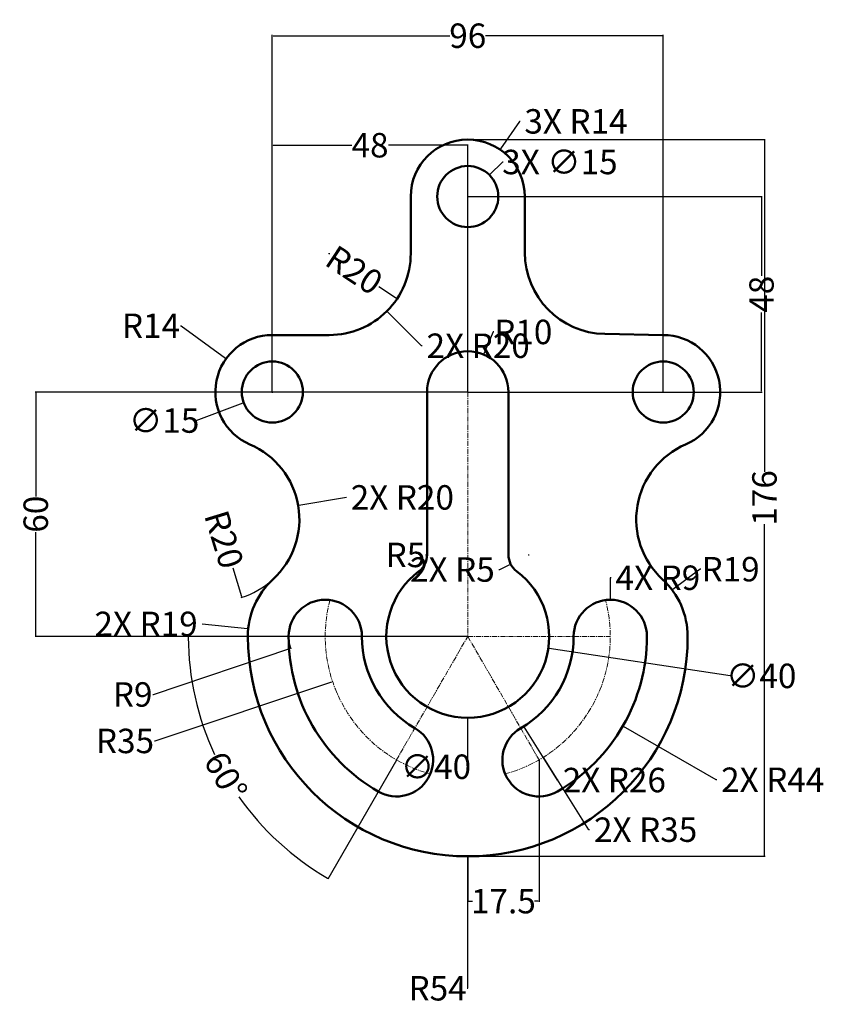
# Model space of a CAD drawing. Units: millimetres. Extents: x 84 to 483, y 14 to 616.
# Tile 1 of 1: x 286.1 to 483.4, y 374.1 to 615.9. Entities that reach past the tile are written whole.
import ezdxf

# ---------------------------------------------------------------- set-up
doc = ezdxf.new("R2010")
doc.units = ezdxf.units.MM
doc.header["$MEASUREMENT"] = 0
doc.linetypes.add('CENTER', pattern=[2, 1.25, -0.25, 0.25, -0.25])
for name, color, linetype, lineweight in [('M-CNTR', 4, 'CENTER', 18), ('M-DIMS', 2, 'Continuous', 25), ('M-OUTL', 7, 'Continuous', 50)]:
    doc.layers.add(name, color=color, linetype=linetype, lineweight=lineweight)
doc.styles.get("Standard").update_dxf_attribs({"font": 'arial.ttf'})
doc.dimstyles.get("Standard").update_dxf_attribs({"dimtxt": 6, "dimasz": 0.18, "dimexe": 0.18, "dimexo": 0.0625, "dimgap": 0.09, "dimtad": 0, "dimtoh": 1, "dimdec": 0, "dimzin": 0, "dimdsep": 46, "dimtxsty": 'Standard', "dimcen": 0.09, "dimadec": 0, "dimazin": 0, "dimtfac": 1, "dimtdec": 0, "dimtofl": 0, "dimtmove": 0, "dimatfit": 3, "dimfxl": 1, "dimtolj": 1, "dimtzin": 0, "dimarcsym": 0})

# ---------------------------------------------------------------- blocks, each defined once
blk = doc.blocks.new('*D1')
at = {"layer": 'Defpoints', "color": 0, "transparency": 16777216}
for p in [(361.12, 464.44), (396.12, 464.44), (396.12, 464.44), (331.63, 440.97), (378.62, 434.13)]:
    blk.add_point(p, dxfattribs=at)
at = {"layer": 'M-DIMS', "color": 0, "lineweight": -2, "transparency": 16777216}
for p, q in [((361.06, 464.44), (327.31, 464.44)), ((378.59, 434.08), (361.72, 404.85))]:
    blk.add_line(p, q, dxfattribs=at)
for start, end in [(180.1503, 204.9914), (215.0086, 239.8497)]:
    blk.add_arc((396.12, 464.44), 68.63, start, end, dxfattribs=at)
at = {"layer": 'M-DIMS', "color": 0, "transparency": 16777216}
for points in [[(327.46, 464.26), (327.52, 464.26), (327.49, 464.44)], [(361.67, 405.12), (361.64, 405.07), (361.81, 405.01)]]:
    blk.add_solid(points, dxfattribs=at)
at = {"layer": 'M-DIMS', "color": 0, "transparency": 16777216, "insert": (336.69, 430.13), "char_height": 6, "attachment_point": 5, "rotation": 300}
blk.add_mtext('\\A1;60°', dxfattribs=at)
blk = doc.blocks.new('*D2')
at = {"layer": 'Defpoints', "color": 0, "transparency": 16777216}
for p in [(444.12, 611.93), (348.12, 524.44), (444.12, 524.44)]:
    blk.add_point(p, dxfattribs=at)
at = {"layer": 'M-DIMS', "color": 0, "lineweight": -2, "transparency": 16777216}
for p, q in [((348.12, 524.5), (348.12, 612.11)), ((348.3, 611.93), (391.74, 611.93)), ((443.94, 611.93), (400.51, 611.93)), ((444.12, 524.5), (444.12, 612.11))]:
    blk.add_line(p, q, dxfattribs=at)
at = {"layer": 'M-DIMS', "color": 0, "transparency": 16777216}
for points in [[(348.3, 611.96), (348.3, 611.9), (348.12, 611.93)], [(443.94, 611.96), (443.94, 611.9), (444.12, 611.93)]]:
    blk.add_solid(points, dxfattribs=at)
at = {"layer": 'M-DIMS', "color": 0, "transparency": 16777216, "insert": (396.12, 611.93), "char_height": 6, "attachment_point": 5}
blk.add_mtext('\\A1;96', dxfattribs=at)
blk = doc.blocks.new('*D3')
at = {"layer": 'Defpoints', "color": 0, "transparency": 16777216}
for p in [(396.12, 524.44), (290.02, 464.44), (396.12, 464.44)]:
    blk.add_point(p, dxfattribs=at)
at = {"layer": 'M-DIMS', "color": 0, "lineweight": -2, "transparency": 16777216}
for p, q in [((396.06, 524.44), (289.84, 524.44)), ((290.02, 524.26), (290.02, 498.83)), ((290.02, 464.62), (290.02, 490.05)), ((396.06, 464.44), (289.84, 464.44))]:
    blk.add_line(p, q, dxfattribs=at)
at = {"layer": 'M-DIMS', "color": 0, "transparency": 16777216}
for points in [[(289.99, 524.26), (290.05, 524.26), (290.02, 524.44)], [(289.99, 464.62), (290.05, 464.62), (290.02, 464.44)]]:
    blk.add_solid(points, dxfattribs=at)
at = {"layer": 'M-DIMS', "color": 0, "transparency": 16777216, "insert": (290.02, 494.44), "char_height": 6, "attachment_point": 5, "rotation": 90}
blk.add_mtext('\\A1;60', dxfattribs=at)
blk = doc.blocks.new('*D4')
at = {"layer": 'Defpoints', "color": 0, "transparency": 16777216}
for p in [(396.12, 572.44), (396.12, 524.44), (468.26, 524.44)]:
    blk.add_point(p, dxfattribs=at)
at = {"layer": 'M-DIMS', "color": 0, "lineweight": -2, "transparency": 16777216}
for p, q in [((396.19, 572.44), (468.44, 572.44)), ((468.26, 572.26), (468.26, 552.96)), ((468.26, 524.62), (468.26, 543.93)), ((396.19, 524.44), (468.44, 524.44))]:
    blk.add_line(p, q, dxfattribs=at)
at = {"layer": 'M-DIMS', "color": 0, "transparency": 16777216}
for points in [[(468.23, 572.26), (468.29, 572.26), (468.26, 572.44)], [(468.23, 524.62), (468.29, 524.62), (468.26, 524.44)]]:
    blk.add_solid(points, dxfattribs=at)
at = {"layer": 'M-DIMS', "color": 0, "transparency": 16777216, "insert": (468.26, 548.44), "char_height": 6, "attachment_point": 5, "rotation": 90}
blk.add_mtext('\\A1;48', dxfattribs=at)
blk = doc.blocks.new('*D5')
at = {"layer": 'Defpoints', "color": 0, "transparency": 16777216}
for p in [(396.12, 585.04), (348.12, 524.44), (396.12, 524.44)]:
    blk.add_point(p, dxfattribs=at)
at = {"layer": 'M-DIMS', "color": 0, "lineweight": -2, "transparency": 16777216}
for p, q in [((348.12, 524.5), (348.12, 585.22)), ((396.12, 524.5), (396.12, 585.22)), ((348.3, 585.04), (367.61, 585.04)), ((395.94, 585.04), (376.64, 585.04))]:
    blk.add_line(p, q, dxfattribs=at)
at = {"layer": 'M-DIMS', "color": 0, "transparency": 16777216}
for points in [[(348.3, 585.07), (348.3, 585.01), (348.12, 585.04)], [(395.94, 585.07), (395.94, 585.01), (396.12, 585.04)]]:
    blk.add_solid(points, dxfattribs=at)
at = {"layer": 'M-DIMS', "color": 0, "transparency": 16777216, "insert": (372.12, 585.04), "char_height": 6, "attachment_point": 5}
blk.add_mtext('\\A1;48', dxfattribs=at)
blk = doc.blocks.new('*D6')
at = {"layer": 'Defpoints', "color": 0, "transparency": 16777216}
for p in [(362.12, 558.44), (378.8, 547.41)]:
    blk.add_point(p, dxfattribs=at)
at = {"layer": 'M-DIMS', "color": 0, "lineweight": -2, "transparency": 16777216}
blk.add_line((374.29, 550.39), (378.65, 547.51), dxfattribs=at)
at = {"layer": 'M-DIMS', "color": 0, "transparency": 16777216}
blk.add_solid([(378.67, 547.53), (378.64, 547.48), (378.8, 547.41)], dxfattribs=at)
at = {"layer": 'M-DIMS', "color": 0, "transparency": 16777216, "insert": (368.25, 554.39), "char_height": 6, "attachment_point": 5, "rotation": 326.5216}
blk.add_mtext('\\A1;R20', dxfattribs=at)
blk = doc.blocks.new('*D7')
at = {"layer": 'Defpoints', "color": 0, "transparency": 16777216}
for p in [(336.8, 532.68), (348.12, 524.44)]:
    blk.add_point(p, dxfattribs=at)
at = {"layer": 'M-DIMS', "color": 0, "lineweight": -2, "transparency": 16777216}
for p, q in [((325.58, 540.71), (325.76, 540.71)), ((325.76, 540.71), (336.66, 532.78)), ((348.03, 524.44), (348.21, 524.44)), ((348.12, 524.35), (348.12, 524.53))]:
    blk.add_line(p, q, dxfattribs=at)
at = {"layer": 'M-DIMS', "color": 0, "transparency": 16777216}
blk.add_solid([(336.67, 532.81), (336.64, 532.76), (336.8, 532.68)], dxfattribs=at)
at = {"layer": 'M-DIMS', "color": 0, "transparency": 16777216, "insert": (318.33, 540.71), "char_height": 6, "attachment_point": 5}
blk.add_mtext('\\A1;R14', dxfattribs=at)
blk = doc.blocks.new('*D8')
at = {"layer": 'Defpoints', "color": 0, "transparency": 16777216}
for p in [(355.15, 527.07), (341.1, 521.81)]:
    blk.add_point(p, dxfattribs=at)
at = {"layer": 'M-DIMS', "color": 0, "lineweight": -2, "transparency": 16777216}
for p, q in [((348.03, 524.44), (348.21, 524.44)), ((348.12, 524.35), (348.12, 524.53)), ((329.42, 517.44), (340.93, 521.75)), ((329.24, 517.44), (329.42, 517.44))]:
    blk.add_line(p, q, dxfattribs=at)
at = {"layer": 'M-DIMS', "color": 0, "transparency": 16777216}
blk.add_solid([(340.92, 521.78), (340.94, 521.72), (341.1, 521.81)], dxfattribs=at)
at = {"layer": 'M-DIMS', "color": 0, "transparency": 16777216, "insert": (321.56, 517.44), "char_height": 6, "attachment_point": 5}
blk.add_mtext('\\A1;∅15', dxfattribs=at)
blk = doc.blocks.new('*D9')
at = {"layer": 'Defpoints', "color": 0, "transparency": 16777216}
for p in [(334.76, 493.18), (340.61, 474.05)]:
    blk.add_point(p, dxfattribs=at)
at = {"layer": 'M-DIMS', "color": 0, "lineweight": -2, "transparency": 16777216}
blk.add_line((338.39, 481.31), (340.56, 474.23), dxfattribs=at)
blk.add_arc((334.76, 493.18), 20, 286.5056, 312.3567, dxfattribs=at)
at = {"layer": 'M-DIMS', "color": 0, "transparency": 16777216}
blk.add_solid([(340.59, 474.24), (340.53, 474.22), (340.61, 474.05)], dxfattribs=at)
at = {"layer": 'M-DIMS', "color": 0, "transparency": 16777216, "insert": (336.27, 488.24), "char_height": 6, "attachment_point": 5, "rotation": 287.0212}
blk.add_mtext('\\A1;R20', dxfattribs=at)
blk = doc.blocks.new('*D10')
at = {"layer": 'Defpoints', "color": 0, "transparency": 16777216}
for p in [(446.34, 475.81), (431.12, 464.44)]:
    blk.add_point(p, dxfattribs=at)
at = {"layer": 'M-DIMS', "color": 0, "lineweight": -2, "transparency": 16777216}
for p, q in [((453.21, 480.94), (446.49, 475.92)), ((453.39, 480.94), (453.21, 480.94)), ((431.03, 464.44), (431.21, 464.44)), ((431.12, 464.35), (431.12, 464.53))]:
    blk.add_line(p, q, dxfattribs=at)
at = {"layer": 'M-DIMS', "color": 0, "transparency": 16777216}
blk.add_solid([(446.47, 475.94), (446.51, 475.9), (446.34, 475.81)], dxfattribs=at)
at = {"layer": 'M-DIMS', "color": 0, "transparency": 16777216, "insert": (460.66, 480.94), "char_height": 6, "attachment_point": 5}
blk.add_mtext('\\A1;R19', dxfattribs=at)
blk = doc.blocks.new('*D11')
at = {"layer": 'Defpoints', "color": 0, "transparency": 16777216}
for p in [(396.12, 464.44), (362.93, 453.34)]:
    blk.add_point(p, dxfattribs=at)
at = {"layer": 'M-DIMS', "color": 0, "lineweight": -2, "transparency": 16777216}
for p, q in [((396.03, 464.44), (396.21, 464.44)), ((396.12, 464.35), (396.12, 464.53)), ((319.39, 438.77), (362.76, 453.28)), ((319.21, 438.77), (319.39, 438.77))]:
    blk.add_line(p, q, dxfattribs=at)
at = {"layer": 'M-DIMS', "color": 0, "transparency": 16777216}
blk.add_solid([(362.75, 453.31), (362.77, 453.25), (362.93, 453.34)], dxfattribs=at)
at = {"layer": 'M-DIMS', "color": 0, "transparency": 16777216, "insert": (311.93, 438.77), "char_height": 6, "attachment_point": 5}
blk.add_mtext('\\A1;R35', dxfattribs=at)
blk = doc.blocks.new('*D12')
at = {"layer": 'Defpoints', "color": 0, "transparency": 16777216}
for p in [(381.12, 484.44), (386.12, 484.44)]:
    blk.add_point(p, dxfattribs=at)
at = {"layer": 'M-DIMS', "color": 0, "lineweight": -2, "transparency": 16777216}
blk.add_line((385.76, 484.44), (385.94, 484.44), dxfattribs=at)
blk.add_arc((381.12, 484.44), 5, 0.7162, 2.0626, dxfattribs=at)
at = {"layer": 'M-DIMS', "color": 0, "transparency": 16777216}
blk.add_solid([(385.94, 484.47), (385.94, 484.41), (386.12, 484.44)], dxfattribs=at)
at = {"layer": 'M-DIMS', "color": 0, "transparency": 16777216, "insert": (380.81, 484.44), "char_height": 6, "attachment_point": 5}
blk.add_mtext('\\A1;R5', dxfattribs=at)
blk = doc.blocks.new('*D13')
at = {"layer": 'Defpoints', "color": 0, "transparency": 16777216}
for p in [(361.12, 464.44), (352.6, 461.56)]:
    blk.add_point(p, dxfattribs=at)
at = {"layer": 'M-DIMS', "color": 0, "lineweight": -2, "transparency": 16777216}
for p, q in [((361.03, 464.44), (361.21, 464.44)), ((361.12, 464.35), (361.12, 464.53)), ((318.94, 450.18), (352.43, 461.5)), ((318.76, 450.18), (318.94, 450.18))]:
    blk.add_line(p, q, dxfattribs=at)
blk.add_arc((361.12, 464.44), 9, 180.3979, 199.8252, dxfattribs=at)
at = {"layer": 'M-DIMS', "color": 0, "transparency": 16777216}
blk.add_solid([(352.42, 461.53), (352.44, 461.47), (352.6, 461.56)], dxfattribs=at)
at = {"layer": 'M-DIMS', "color": 0, "transparency": 16777216, "insert": (313.82, 450.18), "char_height": 6, "attachment_point": 5}
blk.add_mtext('\\A1;R9', dxfattribs=at)
blk = doc.blocks.new('*D14')
at = {"layer": 'Defpoints', "color": 0, "transparency": 16777216}
for p in [(376.35, 467.42), (415.9, 461.46)]:
    blk.add_point(p, dxfattribs=at)
at = {"layer": 'M-DIMS', "color": 0, "lineweight": -2, "transparency": 16777216}
for p, q in [((396.03, 464.44), (396.21, 464.44)), ((396.12, 464.35), (396.12, 464.53)), ((460.55, 454.74), (416.08, 461.44))]:
    blk.add_line(p, q, dxfattribs=at)
at = {"layer": 'M-DIMS', "color": 0, "transparency": 16777216}
blk.add_solid([(416.08, 461.47), (416.07, 461.41), (415.9, 461.46)], dxfattribs=at)
at = {"layer": 'M-DIMS', "color": 0, "transparency": 16777216, "insert": (468.19, 454.74), "char_height": 6, "attachment_point": 5}
blk.add_mtext('\\A1;∅40', dxfattribs=at)
blk = doc.blocks.new('MOUNT-HOLE-D15')
blk.add_circle((7.5, 7.5), 7.5)
blk = doc.blocks.new('*D16')
at = {"layer": 'Defpoints', "color": 0, "transparency": 16777216}
for p in [(396.12, 586.44), (468.98, 586.44), (396.12, 410.44)]:
    blk.add_point(p, dxfattribs=at)
at = {"layer": 'M-DIMS', "color": 0, "lineweight": -2, "transparency": 16777216}
for p, q in [((396.19, 586.44), (469.16, 586.44)), ((468.98, 586.26), (468.98, 504.87)), ((468.98, 410.62), (468.98, 492.01)), ((396.19, 410.44), (469.16, 410.44))]:
    blk.add_line(p, q, dxfattribs=at)
at = {"layer": 'M-DIMS', "color": 0, "transparency": 16777216}
for points in [[(468.95, 586.26), (469.01, 586.26), (468.98, 586.44)], [(468.95, 410.62), (469.01, 410.62), (468.98, 410.44)]]:
    blk.add_solid(points, dxfattribs=at)
at = {"layer": 'M-DIMS', "color": 0, "transparency": 16777216, "insert": (468.98, 498.44), "char_height": 6, "attachment_point": 5, "rotation": 90}
blk.add_mtext('\\A1;176', dxfattribs=at)
blk = doc.blocks.new('*D17')
at = {"layer": 'Defpoints', "color": 0, "transparency": 16777216}
for p in [(413.62, 434.13), (396.12, 410.44), (413.62, 399.44)]:
    blk.add_point(p, dxfattribs=at)
at = {"layer": 'M-DIMS', "color": 0, "lineweight": -2, "transparency": 16777216}
for p, q in [((413.62, 434.07), (413.62, 399.26)), ((396.12, 410.38), (396.12, 399.26)), ((396.3, 399.44), (397.25, 399.44)), ((413.44, 399.44), (412.5, 399.44))]:
    blk.add_line(p, q, dxfattribs=at)
at = {"layer": 'M-DIMS', "color": 0, "transparency": 16777216}
for points in [[(396.3, 399.47), (396.3, 399.41), (396.12, 399.44)], [(413.44, 399.47), (413.44, 399.41), (413.62, 399.44)]]:
    blk.add_solid(points, dxfattribs=at)
at = {"layer": 'M-DIMS', "color": 0, "transparency": 16777216, "insert": (404.87, 399.44), "char_height": 6, "attachment_point": 5}
blk.add_mtext('\\A1;17.5', dxfattribs=at)
blk = doc.blocks.new('*D18')
at = {"layer": 'Defpoints', "color": 0, "transparency": 16777216}
for p in [(401.43, 577.74), (390.82, 567.14)]:
    blk.add_point(p, dxfattribs=at)
at = {"layer": 'M-DIMS', "color": 0, "lineweight": -2, "transparency": 16777216}
for p, q in [((404.61, 580.92), (401.56, 577.87)), ((404.79, 580.92), (404.61, 580.92)), ((396.03, 572.44), (396.21, 572.44)), ((396.12, 572.35), (396.12, 572.53))]:
    blk.add_line(p, q, dxfattribs=at)
at = {"layer": 'M-DIMS', "color": 0, "transparency": 16777216}
blk.add_solid([(401.54, 577.89), (401.58, 577.85), (401.43, 577.74)], dxfattribs=at)
at = {"layer": 'M-DIMS', "color": 0, "transparency": 16777216, "insert": (418.75, 580.92), "char_height": 6, "attachment_point": 5}
blk.add_mtext('\\A1;3X ∅15', dxfattribs=at)
blk = doc.blocks.new('*D19')
at = {"layer": 'Defpoints', "color": 0, "transparency": 16777216}
for p in [(404.06, 583.98), (396.12, 572.44)]:
    blk.add_point(p, dxfattribs=at)
at = {"layer": 'M-DIMS', "color": 0, "lineweight": -2, "transparency": 16777216}
for p, q in [((408.82, 590.9), (404.16, 584.12)), ((409, 590.9), (408.82, 590.9)), ((396.03, 572.44), (396.21, 572.44)), ((396.12, 572.35), (396.12, 572.53))]:
    blk.add_line(p, q, dxfattribs=at)
at = {"layer": 'M-DIMS', "color": 0, "transparency": 16777216}
blk.add_solid([(404.13, 584.14), (404.18, 584.11), (404.06, 583.98)], dxfattribs=at)
at = {"layer": 'M-DIMS', "color": 0, "transparency": 16777216, "insert": (422.69, 590.9), "char_height": 6, "attachment_point": 5}
blk.add_mtext('\\A1;3X R14', dxfattribs=at)
blk = doc.blocks.new('*D20')
at = {"layer": 'Defpoints', "color": 0, "transparency": 16777216}
for p in [(362.12, 558.44), (376.27, 544.3)]:
    blk.add_point(p, dxfattribs=at)
at = {"layer": 'M-DIMS', "color": 0, "lineweight": -2, "transparency": 16777216}
for p, q in [((362.12, 558.35), (362.12, 558.53)), ((362.03, 558.44), (362.21, 558.44)), ((384.75, 535.81), (376.39, 544.17)), ((384.93, 535.81), (384.75, 535.81))]:
    blk.add_line(p, q, dxfattribs=at)
at = {"layer": 'M-DIMS', "color": 0, "transparency": 16777216}
blk.add_solid([(376.41, 544.19), (376.37, 544.15), (376.27, 544.3)], dxfattribs=at)
at = {"layer": 'M-DIMS', "color": 0, "transparency": 16777216, "insert": (398.68, 535.81), "char_height": 6, "attachment_point": 5}
blk.add_mtext('\\A1;2X R20', dxfattribs=at)
blk = doc.blocks.new('*D21')
at = {"layer": 'Defpoints', "color": 0, "transparency": 16777216}
for p in [(354.47, 496.55), (334.76, 493.18)]:
    blk.add_point(p, dxfattribs=at)
at = {"layer": 'M-DIMS', "color": 0, "lineweight": -2, "transparency": 16777216}
for p, q in [((366.3, 498.57), (354.65, 496.58)), ((334.76, 493.09), (334.76, 493.27)), ((334.67, 493.18), (334.85, 493.18))]:
    blk.add_line(p, q, dxfattribs=at)
at = {"layer": 'M-DIMS', "color": 0, "transparency": 16777216}
blk.add_solid([(354.64, 496.61), (354.65, 496.55), (354.47, 496.55)], dxfattribs=at)
at = {"layer": 'M-DIMS', "color": 0, "transparency": 16777216, "insert": (380.05, 498.57), "char_height": 6, "attachment_point": 5}
blk.add_mtext('\\A1;2X R20', dxfattribs=at)
blk = doc.blocks.new('*D22')
at = {"layer": 'Defpoints', "color": 0, "transparency": 16777216}
for p in [(342.22, 466.36), (361.12, 464.44)]:
    blk.add_point(p, dxfattribs=at)
at = {"layer": 'M-DIMS', "color": 0, "lineweight": -2, "transparency": 16777216}
for p, q in [((330.88, 467.51), (342.04, 466.38)), ((361.03, 464.44), (361.21, 464.44)), ((361.12, 464.35), (361.12, 464.53))]:
    blk.add_line(p, q, dxfattribs=at)
at = {"layer": 'M-DIMS', "color": 0, "transparency": 16777216}
blk.add_solid([(342.04, 466.41), (342.04, 466.35), (342.22, 466.36)], dxfattribs=at)
at = {"layer": 'M-DIMS', "color": 0, "transparency": 16777216, "insert": (317.12, 467.51), "char_height": 6, "attachment_point": 5}
blk.add_mtext('\\A1;2X R19', dxfattribs=at)
blk = doc.blocks.new('*D23')
at = {"layer": 'Defpoints', "color": 0, "transparency": 16777216}
for p in [(396.12, 464.44), (396.12, 410.44)]:
    blk.add_point(p, dxfattribs=at)
at = {"layer": 'M-DIMS', "color": 0, "lineweight": -2, "transparency": 16777216}
for p, q in [((396.03, 464.44), (396.21, 464.44)), ((396.12, 464.35), (396.12, 464.53)), ((396.12, 378.04), (396.12, 410.26)), ((395.94, 378.04), (396.12, 378.04))]:
    blk.add_line(p, q, dxfattribs=at)
at = {"layer": 'M-DIMS', "color": 0, "transparency": 16777216}
blk.add_solid([(396.09, 410.26), (396.15, 410.26), (396.12, 410.44)], dxfattribs=at)
at = {"layer": 'M-DIMS', "color": 0, "transparency": 16777216, "insert": (388.7, 378.04), "char_height": 6, "attachment_point": 5}
blk.add_mtext('\\A1;R54', dxfattribs=at)
blk = doc.blocks.new('*D24')
at = {"layer": 'Defpoints', "color": 0, "transparency": 16777216}
for p in [(400, 533.66), (396.12, 524.44)]:
    blk.add_point(p, dxfattribs=at)
at = {"layer": 'M-DIMS', "color": 0, "lineweight": -2, "transparency": 16777216}
for p, q in [((402.33, 539.19), (400.07, 533.82)), ((402.51, 539.19), (402.33, 539.19)), ((396.03, 524.44), (396.21, 524.44)), ((396.12, 524.35), (396.12, 524.53))]:
    blk.add_line(p, q, dxfattribs=at)
at = {"layer": 'M-DIMS', "color": 0, "transparency": 16777216}
blk.add_solid([(400.04, 533.84), (400.1, 533.81), (400, 533.66)], dxfattribs=at)
at = {"layer": 'M-DIMS', "color": 0, "transparency": 16777216, "insert": (409.75, 539.19), "char_height": 6, "attachment_point": 5}
blk.add_mtext('\\A1;R10', dxfattribs=at)
blk = doc.blocks.new('*D25')
at = {"layer": 'Defpoints', "color": 0, "transparency": 16777216}
for p in [(411.12, 484.44), (406.65, 482.2)]:
    blk.add_point(p, dxfattribs=at)
at = {"layer": 'M-DIMS', "color": 0, "lineweight": -2, "transparency": 16777216}
for p, q in [((411.03, 484.44), (411.21, 484.44)), ((411.12, 484.35), (411.12, 484.53)), ((403.97, 480.86), (406.49, 482.12)), ((403.79, 480.86), (403.97, 480.86))]:
    blk.add_line(p, q, dxfattribs=at)
at = {"layer": 'M-DIMS', "color": 0, "transparency": 16777216}
blk.add_solid([(406.48, 482.15), (406.5, 482.1), (406.65, 482.2)], dxfattribs=at)
at = {"layer": 'M-DIMS', "color": 0, "transparency": 16777216, "insert": (392.34, 480.86), "char_height": 6, "attachment_point": 5}
blk.add_mtext('\\A1;2X R5', dxfattribs=at)
blk = doc.blocks.new('*D26')
at = {"layer": 'Defpoints', "color": 0, "transparency": 16777216}
for p in [(396.12, 484.44), (396.12, 444.44)]:
    blk.add_point(p, dxfattribs=at)
at = {"layer": 'M-DIMS', "color": 0, "lineweight": -2, "transparency": 16777216}
for p, q in [((396.03, 464.44), (396.21, 464.44)), ((396.12, 464.35), (396.12, 464.53)), ((396.12, 432.44), (396.12, 444.26)), ((395.94, 432.44), (396.12, 432.44))]:
    blk.add_line(p, q, dxfattribs=at)
at = {"layer": 'M-DIMS', "color": 0, "transparency": 16777216}
blk.add_solid([(396.09, 444.26), (396.15, 444.26), (396.12, 444.44)], dxfattribs=at)
at = {"layer": 'M-DIMS', "color": 0, "transparency": 16777216, "insert": (388.3, 432.44), "char_height": 6, "attachment_point": 5}
blk.add_mtext('\\A1;∅40', dxfattribs=at)
blk = doc.blocks.new('*D27')
at = {"layer": 'Defpoints', "color": 0, "transparency": 16777216}
for p in [(431.12, 473.44), (431.12, 464.44)]:
    blk.add_point(p, dxfattribs=at)
at = {"layer": 'M-DIMS', "color": 0, "lineweight": -2, "transparency": 16777216}
for p, q in [((431.3, 478.84), (431.12, 478.84)), ((431.12, 478.84), (431.12, 473.62)), ((431.03, 464.44), (431.21, 464.44)), ((431.12, 464.35), (431.12, 464.53))]:
    blk.add_line(p, q, dxfattribs=at)
at = {"layer": 'M-DIMS', "color": 0, "transparency": 16777216}
blk.add_solid([(431.09, 473.62), (431.15, 473.62), (431.12, 473.44)], dxfattribs=at)
at = {"layer": 'M-DIMS', "color": 0, "transparency": 16777216, "insert": (442.8, 478.84), "char_height": 6, "attachment_point": 5}
blk.add_mtext('\\A1;4X R9', dxfattribs=at)
blk = doc.blocks.new('*D28')
at = {"layer": 'Defpoints', "color": 0, "transparency": 16777216}
for p in [(396.12, 464.44), (434.23, 442.44)]:
    blk.add_point(p, dxfattribs=at)
at = {"layer": 'M-DIMS', "color": 0, "lineweight": -2, "transparency": 16777216}
for p, q in [((396.03, 464.44), (396.21, 464.44)), ((396.12, 464.35), (396.12, 464.53)), ((457.09, 429.24), (434.38, 442.35)), ((457.27, 429.24), (457.09, 429.24))]:
    blk.add_line(p, q, dxfattribs=at)
at = {"layer": 'M-DIMS', "color": 0, "transparency": 16777216}
blk.add_solid([(434.4, 442.38), (434.37, 442.32), (434.23, 442.44)], dxfattribs=at)
at = {"layer": 'M-DIMS', "color": 0, "transparency": 16777216, "insert": (471.01, 429.24), "char_height": 6, "attachment_point": 5}
blk.add_mtext('\\A1;2X R44', dxfattribs=at)
blk = doc.blocks.new('*D29')
at = {"layer": 'Defpoints', "color": 0, "transparency": 16777216}
for p in [(396.12, 464.44), (414.7, 434.78)]:
    blk.add_point(p, dxfattribs=at)
at = {"layer": 'M-DIMS', "color": 0, "lineweight": -2, "transparency": 16777216}
for p, q in [((396.03, 464.44), (396.21, 464.44)), ((396.12, 464.35), (396.12, 464.53)), ((425.84, 416.98), (414.79, 434.62)), ((426.02, 416.98), (425.84, 416.98))]:
    blk.add_line(p, q, dxfattribs=at)
at = {"layer": 'M-DIMS', "color": 0, "transparency": 16777216}
blk.add_solid([(414.82, 434.64), (414.77, 434.61), (414.7, 434.78)], dxfattribs=at)
at = {"layer": 'M-DIMS', "color": 0, "transparency": 16777216, "insert": (439.8, 416.98), "char_height": 6, "attachment_point": 5}
blk.add_mtext('\\A1;2X R35', dxfattribs=at)
blk = doc.blocks.new('*D30')
at = {"layer": 'Defpoints', "color": 0, "transparency": 16777216}
for p in [(396.12, 464.44), (409.9, 442.39)]:
    blk.add_point(p, dxfattribs=at)
at = {"layer": 'M-DIMS', "color": 0, "lineweight": -2, "transparency": 16777216}
for p, q in [((396.03, 464.44), (396.21, 464.44)), ((396.12, 464.35), (396.12, 464.53)), ((418.17, 429.17), (410, 442.24)), ((418.35, 429.17), (418.17, 429.17))]:
    blk.add_line(p, q, dxfattribs=at)
at = {"layer": 'M-DIMS', "color": 0, "transparency": 16777216}
blk.add_solid([(410.02, 442.26), (409.97, 442.23), (409.9, 442.39)], dxfattribs=at)
at = {"layer": 'M-DIMS', "color": 0, "transparency": 16777216, "insert": (432.11, 429.17), "char_height": 6, "attachment_point": 5}
blk.add_mtext('\\A1;2X R26', dxfattribs=at)

msp = doc.modelspace()

# ---------------------------------------------------------------- linework, layer by layer
at = {"layer": 'M-CNTR'}
msp.add_line((406.12, 524.44), (406.12, 497.98), dxfattribs=at)
for points in [[(396.12, 572.44), (396.12, 524.44), (444.12, 524.44)], [(348.12, 524.44), (396.12, 524.44), (396.12, 464.44)], [(361.12, 464.44), (396.12, 464.44), (431.12, 464.44)], [(378.62, 434.13), (396.12, 464.44), (413.62, 434.13)]]:
    msp.add_lwpolyline(points, dxfattribs=at)
for start, end in [(165.2259, 254.7741), (285.2259, 14.7741)]:
    msp.add_arc((396.12, 464.44), 35, start, end, dxfattribs=at)
at = {"layer": 'M-OUTL'}
for points in [[(450.12, 464.44, -1), (342.12, 464.44, -0.210115), (348.28, 478.44, 0.544741), (342.62, 511.57, -0.815954), (348.12, 538.44), (362.12, 538.44, 0.414214), (382.12, 558.44), (382.12, 572.44, -1), (410.12, 572.44), (410.12, 558.7, 0.408916), (429.76, 538.7), (444.12, 538.44, -0.815954), (449.63, 511.57, 0.544741), (443.97, 478.44, -0.210115)], [(406.12, 484.44, 0.236068), (408.12, 480.44, -3), (384.12, 480.44, 0.236068), (386.12, 484.44), (386.12, 524.44, -1), (406.12, 524.44)], [(374.12, 426.34, 1), (383.12, 441.92, -0.267949), (370.12, 464.44, 1), (352.12, 464.44, 0.267949)], [(440.12, 464.44, 1), (422.12, 464.44, -0.267949), (409.12, 441.92, 1), (418.12, 426.34, 0.267949)]]:
    msp.add_lwpolyline(points, format="xyb", close=True, dxfattribs=at)

# ---------------------------------------------------------------- block references
for p in [(388.62, 564.94), (340.62, 516.94), (436.62, 516.94)]:
    msp.add_blockref('MOUNT-HOLE-D15', p, dxfattribs=at)

# ---------------------------------------------------------------- dimensions: what is measured, and where the dimension line sits
at = {"layer": 'M-DIMS'}
for base, p1, p2, override, picture, middle in [((444.12, 611.93), (348.12, 524.44), (444.12, 524.44), {"dimclrd": 0, "dimclre": 0, "dimclrt": 0}, '*D2', (396.12, 611.93)), ((396.12, 585.04), (348.12, 524.44), (396.12, 524.44), {"dimclrd": 0, "dimclre": 0, "dimclrt": 0}, '*D5', (372.12, 585.04)), ((413.62, 399.44), (396.12, 410.44), (413.62, 434.13), {"dimdec": 1, "dimlfac": 1, "dimrnd": 0, "dimzin": 0, "dimdsep": 46, "dimlunit": 2}, '*D17', (404.87, 399.44))]:
    dim = msp.add_linear_dim(base=base, p1=p1, p2=p2, dimstyle='Standard', override=override, dxfattribs=at)
    dim.commit()
    dim.dimension.update_dxf_attribs({"geometry": picture, "text_midpoint": middle})
for center, mpoint, text, picture, middle in [((396.12, 572.44), (404.06, 583.98), '3X <>', '*D19', (422.69, 590.9)), ((362.12, 558.44), (376.27, 544.3), '2X <>', '*D20', (398.68, 535.81)), ((334.76, 493.18), (354.47, 496.55), '2X <>', '*D21', (366.3, 498.57)), ((411.12, 484.44), (406.65, 482.2), '2X <>', '*D25', (392.34, 480.86)), ((431.12, 464.44), (431.12, 473.44), '4X <>', '*D27', (442.8, 478.84)), ((361.12, 464.44), (342.22, 466.36), '2X <>', '*D22', (330.88, 467.51)), ((396.12, 464.44), (434.23, 442.44), '2X <>', '*D28', (471.01, 429.24)), ((396.12, 464.44), (414.7, 434.78), '2X <>', '*D29', (439.8, 416.98)), ((396.12, 464.44), (409.9, 442.39), '2X <>', '*D30', (432.11, 429.17))]:
    dim = msp.add_radius_dim(center=center, mpoint=mpoint, text=text, dimstyle='Standard', override={"dimdec": 0, "dimlfac": 1, "dimrnd": 0, "dimzin": 0, "dimdsep": 46, "dimlunit": 2}, dxfattribs=at)
    dim.commit()
    dim.dimension.update_dxf_attribs({"geometry": picture, "text_midpoint": middle, "dimtype": 164})
dim = msp.add_diameter_dim_2p(p1=(390.82, 567.14), p2=(401.43, 577.74), text='3X <>', dimstyle='Standard', override={"dimdec": 0, "dimlfac": 1, "dimrnd": 0, "dimzin": 0, "dimdsep": 46, "dimlunit": 2}, dxfattribs=at)
dim.commit()
dim.dimension.update_dxf_attribs({"geometry": '*D18', "text_midpoint": (418.75, 580.92), "dimtype": 163})
for base, p1, p2, override, picture, middle in [((468.98, 586.44), (396.12, 410.44), (396.12, 586.44), {"dimdec": 0, "dimlfac": 1, "dimrnd": 0, "dimzin": 0, "dimdsep": 46, "dimlunit": 2}, '*D16', (468.98, 498.44)), ((468.26, 524.44), (396.12, 572.44), (396.12, 524.44), {"dimclrd": 0, "dimclre": 0, "dimclrt": 0}, '*D4', (468.26, 548.44)), ((290.02, 464.44), (396.12, 524.44), (396.12, 464.44), {"dimclrd": 0, "dimclre": 0, "dimclrt": 0}, '*D3', (290.02, 494.44))]:
    dim = msp.add_linear_dim(base=base, p1=p1, p2=p2, angle=90, dimstyle='Standard', override=override, dxfattribs=at)
    dim.commit()
    dim.dimension.update_dxf_attribs({"geometry": picture, "text_midpoint": middle})
for center, mpoint, override, picture, middle in [((362.12, 558.44), (378.8, 547.41), {"dimclrd": 0, "dimclre": 0, "dimclrt": 0}, '*D6', (368.25, 554.39)), ((348.12, 524.44), (336.8, 532.68), {"dimclrd": 0, "dimclre": 0, "dimclrt": 0}, '*D7', (318.33, 540.71)), ((396.12, 524.44), (400, 533.66), {"dimdec": 0, "dimlfac": 1, "dimrnd": 0, "dimzin": 0, "dimdsep": 46, "dimlunit": 2}, '*D24', (409.75, 539.19)), ((334.76, 493.18), (340.61, 474.05), {"dimclrd": 0, "dimclre": 0, "dimclrt": 0}, '*D9', (336.27, 488.24)), ((381.12, 484.44), (386.12, 484.44), {"dimclrd": 0, "dimclre": 0, "dimclrt": 0}, '*D12', (380.81, 484.44)), ((431.12, 464.44), (446.34, 475.81), {"dimclrd": 0, "dimclre": 0, "dimclrt": 0}, '*D10', (460.66, 480.94)), ((396.12, 464.44), (362.93, 453.34), {"dimclrd": 0, "dimclre": 0, "dimclrt": 0}, '*D11', (311.93, 438.77)), ((361.12, 464.44), (352.6, 461.56), {"dimclrd": 0, "dimclre": 0, "dimclrt": 0}, '*D13', (313.82, 450.18)), ((396.12, 464.44), (396.12, 410.44), {"dimdec": 0, "dimlfac": 1, "dimrnd": 0, "dimzin": 0, "dimdsep": 46, "dimlunit": 2}, '*D23', (388.7, 378.04))]:
    dim = msp.add_radius_dim(center=center, mpoint=mpoint, dimstyle='Standard', override=override, dxfattribs=at)
    dim.commit()
    dim.dimension.update_dxf_attribs({"geometry": picture, "text_midpoint": middle, "dimtype": 164})
for p1, p2, override, picture, middle in [((355.15, 527.07), (341.1, 521.81), {"dimclrd": 0, "dimclre": 0, "dimclrt": 0}, '*D8', (321.56, 517.44)), ((396.12, 484.44), (396.12, 444.44), {"dimdec": 0, "dimlfac": 1, "dimrnd": 0, "dimzin": 0, "dimdsep": 46, "dimlunit": 2}, '*D26', (388.3, 432.44)), ((376.35, 467.42), (415.9, 461.46), {"dimclrd": 0, "dimclre": 0, "dimclrt": 0}, '*D14', (460.55, 454.74))]:
    dim = msp.add_diameter_dim_2p(p1=p1, p2=p2, dimstyle='Standard', override=override, dxfattribs=at)
    dim.commit()
    dim.dimension.update_dxf_attribs({"geometry": picture, "text_midpoint": middle, "dimtype": 163})
dim = msp.add_angular_dim_2l(base=(331.63, 440.97), line1=((396.12, 464.44), (378.62, 434.13)), line2=((396.12, 464.44), (361.12, 464.44)), dimstyle='Standard', override={"dimclrd": 0, "dimclre": 0, "dimclrt": 0}, dxfattribs=at)
dim.commit()
dim.dimension.update_dxf_attribs({"geometry": '*D1', "text_midpoint": (336.69, 430.13)})

doc.saveas('drawing.dxf')
